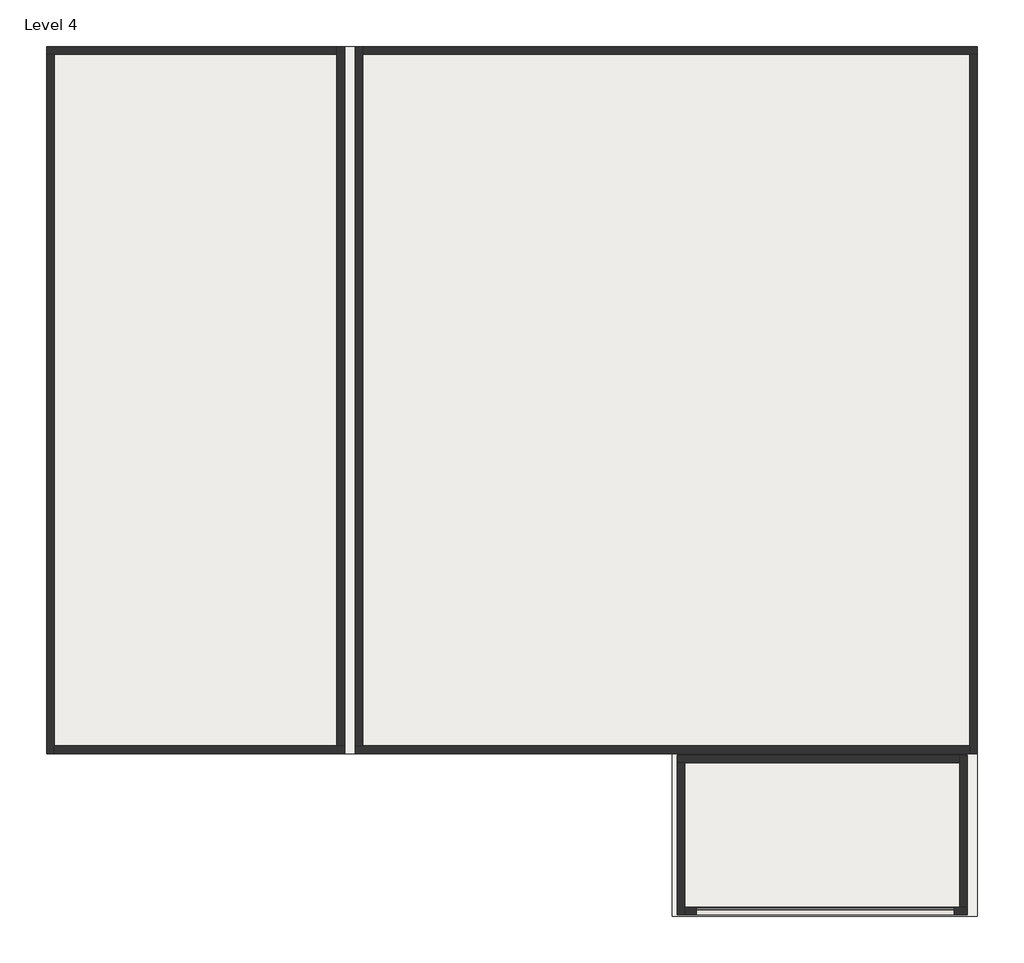
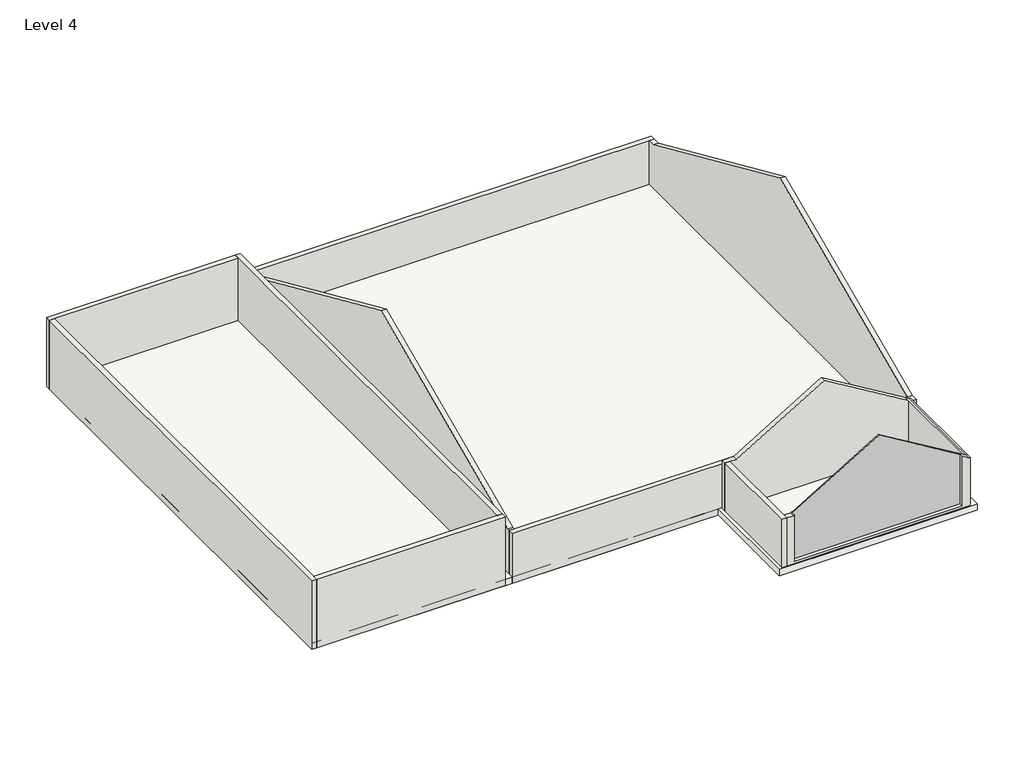
# One storey: 12 walls, 1 plate, 1 slab.
"""IFC4 building model written with IfcOpenShell, lengths in millimetres."""

from ifc_helpers import new_model, si_unit, frame, origin, place, context, project, spatial, polyline, outline, extrude, faceted_brep, transform, mapped, element, save
from components import system_panel_glazed_24e5f3e2

model = new_model("IFC4")

# Units and contexts
model_context = context("Model", 3, world=origin())
ifc_project = project(units=[si_unit("LENGTHUNIT", "METRE", prefix="MILLI")], contexts=[model_context])

# Site, building, storey
site = spatial("IfcSite", under=ifc_project)
building = spatial("IfcBuilding", under=site)
storey = spatial("IfcBuildingStorey", under=building, Name="Level 4", Elevation=6858.0)

# Plate
placement = place(None, origin())
system_panel_glazed_shape = system_panel_glazed_24e5f3e2(model_context)
element("IfcPlate", 1, ObjectType="System Panel : Glazed", at=placement, inside=storey, context=model_context, shape_type="MappedRepresentation", body=[
    mapped(system_panel_glazed_shape, transform((5277.9635732, -1650.5734736, 7068.8144542), x_axis=(1.0, 0.0, 0.0), y_axis=(0.0, 1.0, 0.0), z_axis=(0.0, 0.0, 1.0))),
])

# Slab
element("IfcSlab", 2, ObjectType="6\" GF", at=placement, inside=storey, context=model_context, shape_type="SweptSolid", body=[
    extrude(outline(polyline([(-6386.9864268, 11297.0765264), (7557.6135732, 11297.0765264), (7557.6135732, -1733.1234736), (2985.6135732, -1733.1234736), (2985.6135732, 705.2765264), (365.6851234, 705.2765264), (-6386.9864268, 705.2765264), (-6386.9864268, 11297.0765264)])), frame((0.0, 0.0, 6858.0), z_axis=(0.0, 0.0, 1.0), x_axis=(1.0, 0.0, 0.0)), (0.0, 0.0, 1.0), 152.4),
])

# Walls
element("IfcWall", 3, ObjectType="4.5\" wall", at=placement, inside=storey, context=model_context, shape_type="Brep", body=[
    faceted_brep([(7405.2135732, -1593.4234736, 6858.0), (7290.9135732, -1593.4234736, 6858.0), (3176.1135732, -1593.4234736, 6858.0), (3176.1135732, -1593.4234736, 8183.7639477), (3326.968548, -1593.4234736, 8183.7639477), (3347.5635732, -1593.4234736, 8196.1386873), (3347.5635732, -1593.4234736, 7068.8144542), (7208.3635732, -1593.4234736, 7068.8144542), (7208.3635732, -1593.4234736, 8280.0789158), (7290.9135732, -1593.4234736, 8230.4778717), (7368.6585985, -1593.4234736, 8183.7639477), (7405.2135732, -1593.4234736, 8183.7639477), (3176.1135732, -1707.7234736, 6858.0), (7405.2135732, -1707.7234736, 6858.0), (7405.2135732, -1707.7234736, 8183.7639477), (7368.6585985, -1707.7234736, 8183.7639477), (7208.3635732, -1707.7234736, 8280.0789158), (7208.3635732, -1707.7234736, 7068.8144542), (3347.5635732, -1707.7234736, 7068.8144542), (3347.5635732, -1707.7234736, 8196.1386873), (3326.968548, -1707.7234736, 8183.7639477), (3176.1135732, -1707.7234736, 8183.7639477)], [[[0, 1, 2, 3, 4, 5, 6, 7, 8, 9, 10, 11]], [[12, 13, 14, 15, 16, 17, 18, 19, 20, 21]], [[2, 1, 0, 13, 12]], [[0, 11, 14, 13]], [[3, 2, 12, 21]], [[14, 11, 10, 15]], [[15, 10, 9, 8, 16]], [[4, 20, 19, 5]], [[3, 21, 20, 4]], [[18, 6, 5, 19]], [[7, 17, 16, 8]], [[6, 18, 17, 7]]]),
])
element("IfcWall", 4, ObjectType="4.5\" wall", at=placement, inside=storey, context=model_context, shape_type="Brep", body=[
    faceted_brep([(7290.9135732, 679.8765264, 6858.0), (7290.9135732, 565.5765264, 6858.0), (7290.9135732, -1593.4234736, 6858.0), (7290.9135732, -1593.4234736, 8230.4778717), (7290.9135732, 565.5765264, 8230.4778717), (7290.9135732, 679.8765264, 8230.4778717), (7405.2135732, 679.8765264, 6858.0), (7405.2135732, 679.8765264, 8183.7639477), (7405.2135732, -1593.4234736, 8183.7639477), (7405.2135732, -1593.4234736, 6858.0), (7368.6585985, 679.8765264, 8183.7639477), (7368.6585985, -1593.4234736, 8183.7639477)], [[[0, 1, 2, 3, 4, 5]], [[6, 7, 8, 9]], [[2, 1, 0, 6, 9]], [[0, 5, 10, 7, 6]], [[3, 2, 9, 8, 11]], [[5, 4, 3, 11, 10]], [[11, 8, 7, 10]]]),
])
element("IfcWall", 5, ObjectType="4.5\" wall", at=placement, inside=storey, context=model_context, shape_type="Brep", body=[
    faceted_brep([(3061.8135732, 565.5765264, 6858.0), (3176.1135732, 565.5765264, 6858.0), (7290.9135732, 565.5765264, 6858.0), (7290.9135732, 565.5765264, 8230.4778717), (5347.8135732, 565.5765264, 9398.0101405), (3326.968548, 565.5765264, 8183.7639477), (3176.1135732, 565.5765264, 8183.7639477), (3061.8135732, 565.5765264, 8183.7639477), (3061.8135732, 679.8765264, 6858.0), (3061.8135732, 679.8765264, 8183.7639477), (3326.968548, 679.8765264, 8183.7639477), (5347.8135732, 679.8765264, 9398.0101405), (7290.9135732, 679.8765264, 8230.4778717), (7290.9135732, 679.8765264, 6858.0)], [[[0, 1, 2, 3, 4, 5, 6, 7]], [[8, 9, 10, 11, 12, 13]], [[2, 1, 0, 8, 13]], [[0, 7, 9, 8]], [[3, 2, 13, 12]], [[7, 6, 5, 10, 9]], [[5, 4, 11, 10]], [[4, 3, 12, 11]]]),
])
element("IfcWall", 6, ObjectType="4.5\" wall", at=placement, inside=storey, context=model_context, shape_type="Brep", body=[
    faceted_brep([(3176.1135732, -1707.7234736, 6858.0), (3176.1135732, -1593.4234736, 6858.0), (3176.1135732, 565.5765264, 6858.0), (3176.1135732, 565.5765264, 8183.7639477), (3176.1135732, -1593.4234736, 8183.7639477), (3176.1135732, -1707.7234736, 8183.7639477), (3061.8135732, -1707.7234736, 6858.0), (3061.8135732, -1707.7234736, 8183.7639477), (3061.8135732, 565.5765264, 8183.7639477), (3061.8135732, 565.5765264, 6858.0)], [[[0, 1, 2, 3, 4, 5]], [[6, 7, 8, 9]], [[2, 1, 0, 6, 9]], [[0, 5, 7, 6]], [[3, 2, 9, 8]], [[5, 4, 3, 8, 7]]]),
])
element("IfcWall", 7, ObjectType="4.5\" wall", at=placement, inside=storey, context=model_context, shape_type="Brep", body=[
    faceted_brep([(7557.6135732, 11297.0765264, 6858.0), (-1648.9651673, 11297.0765264, 6858.0), (-1648.9651673, 11297.0765264, 8077.2), (7557.6135732, 11297.0765264, 8077.2), (7557.6135732, 11182.7765264, 6858.0), (7557.6135732, 11182.7765264, 8077.2), (7443.3135732, 11182.7765264, 8077.2), (-1648.9651673, 11182.7765264, 8077.2), (-1648.9651673, 11182.7765264, 6858.0), (7443.3135732, 11182.7765264, 6858.0)], [[[0, 1, 2, 3]], [[4, 5, 6, 7, 8, 9]], [[1, 0, 4, 9, 8]], [[3, 2, 7, 6, 5]], [[0, 3, 5, 4]], [[2, 1, 8, 7]]]),
])
element("IfcWall", 8, ObjectType="4.5\" wall", at=placement, inside=storey, context=model_context, shape_type="Brep", body=[
    faceted_brep([(7557.6135732, 705.2765264, 6858.0), (7557.6135732, 11182.7765264, 6858.0), (7557.6135732, 11182.7765264, 8077.2), (7557.6135732, 11013.6793515, 8077.2), (7557.6135732, 5944.0265264, 10334.3548623), (7557.6135732, 874.3737012, 8077.2), (7557.6135732, 705.2765264, 8077.2), (7443.3135732, 705.2765264, 6858.0), (7443.3135732, 705.2765264, 8077.2), (7443.3135732, 819.5765264, 8077.2), (7443.3135732, 874.3737012, 8077.2), (7443.3135732, 5944.0265264, 10334.3548623), (7443.3135732, 11013.6793515, 8077.2), (7443.3135732, 11182.7765264, 8077.2), (7443.3135732, 11182.7765264, 6858.0), (7443.3135732, 819.5765264, 6858.0)], [[[0, 1, 2, 3, 4, 5, 6]], [[7, 8, 9, 10, 11, 12, 13, 14, 15]], [[1, 0, 7, 15, 14]], [[0, 6, 8, 7]], [[2, 1, 14, 13]], [[6, 5, 10, 9, 8]], [[5, 4, 11, 10]], [[4, 3, 12, 11]], [[3, 2, 13, 12]]]),
])
element("IfcWall", 9, ObjectType="4.5\" wall", at=placement, inside=storey, context=model_context, shape_type="Brep", body=[
    faceted_brep([(-1763.2651673, 705.2765264, 6858.0), (7443.3135732, 705.2765264, 6858.0), (7443.3135732, 705.2765264, 8077.2), (-1763.2651673, 705.2765264, 8077.2), (-1763.2651673, 819.5765264, 6858.0), (-1763.2651673, 819.5765264, 8077.2), (-1648.9651673, 819.5765264, 8077.2), (7443.3135732, 819.5765264, 8077.2), (7443.3135732, 819.5765264, 6858.0), (-1648.9651673, 819.5765264, 6858.0)], [[[0, 1, 2, 3]], [[4, 5, 6, 7, 8, 9]], [[1, 0, 4, 9, 8]], [[3, 2, 7, 6, 5]], [[0, 3, 5, 4]], [[2, 1, 8, 7]]]),
])
element("IfcWall", 10, ObjectType="4.5\" wall", at=placement, inside=storey, context=model_context, shape_type="Brep", body=[
    faceted_brep([(-1763.2651673, 11297.0765264, 6858.0), (-1763.2651673, 819.5765264, 6858.0), (-1763.2651673, 819.5765264, 8077.2), (-1763.2651673, 874.3737012, 8077.2), (-1763.2651673, 5944.0265264, 10334.3548623), (-1763.2651673, 11013.6793515, 8077.2), (-1763.2651673, 11297.0765264, 8077.2), (-1648.9651673, 11297.0765264, 6858.0), (-1648.9651673, 11297.0765264, 8077.2), (-1648.9651673, 11182.7765264, 8077.2), (-1648.9651673, 11013.6793515, 8077.2), (-1648.9651673, 5944.0265264, 10334.3548623), (-1648.9651673, 874.3737012, 8077.2), (-1648.9651673, 819.5765264, 8077.2), (-1648.9651673, 819.5765264, 6858.0), (-1648.9651673, 11182.7765264, 6858.0)], [[[0, 1, 2, 3, 4, 5, 6]], [[7, 8, 9, 10, 11, 12, 13, 14, 15]], [[1, 0, 7, 15, 14]], [[0, 6, 8, 7]], [[2, 1, 14, 13]], [[6, 5, 10, 9, 8]], [[5, 4, 11, 10]], [[4, 3, 12, 11]], [[3, 2, 13, 12]]]),
])
element("IfcWall", 11, ObjectType="4.5\" wall", at=placement, inside=storey, context=model_context, shape_type="Brep", body=[
    faceted_brep([(-6386.9864268, 11182.7765264, 6858.0), (-6272.6864268, 11182.7765264, 6858.0), (-2037.3924436, 11182.7765264, 6858.0), (-2037.3924436, 11182.7765264, 8533.9641574), (-6272.6864268, 11182.7765264, 8533.9641574), (-6386.9864268, 11182.7765264, 8533.9641574), (-6386.9864268, 11297.0765264, 6858.0), (-6386.9864268, 11297.0765264, 8533.9641574), (-2037.3924436, 11297.0765264, 8533.9641574), (-2037.3924436, 11297.0765264, 6858.0)], [[[0, 1, 2, 3, 4, 5]], [[6, 7, 8, 9]], [[2, 1, 0, 6, 9]], [[5, 4, 3, 8, 7]], [[0, 5, 7, 6]], [[3, 2, 9, 8]]]),
])
element("IfcWall", 12, ObjectType="4.5\" wall", at=placement, inside=storey, context=model_context, shape_type="Brep", body=[
    faceted_brep([(-6272.6864268, 705.2765264, 6858.0), (-6272.6864268, 819.5765264, 6858.0), (-6272.6864268, 11182.7765264, 6858.0), (-6272.6864268, 11182.7765264, 8533.9641574), (-6272.6864268, 819.5765264, 8533.9641574), (-6272.6864268, 705.2765264, 8533.9641574), (-6386.9864268, 705.2765264, 6858.0), (-6386.9864268, 705.2765264, 8533.9641574), (-6386.9864268, 11182.7765264, 8533.9641574), (-6386.9864268, 11182.7765264, 6858.0)], [[[0, 1, 2, 3, 4, 5]], [[6, 7, 8, 9]], [[2, 1, 0, 6, 9]], [[5, 4, 3, 8, 7]], [[0, 5, 7, 6]], [[3, 2, 9, 8]]]),
])
element("IfcWall", 13, ObjectType="4.5\" wall", at=placement, inside=storey, context=model_context, shape_type="Brep", body=[
    faceted_brep([(-1923.0924436, 819.5765264, 6858.0), (-2037.3924436, 819.5765264, 6858.0), (-6272.6864268, 819.5765264, 6858.0), (-6272.6864268, 819.5765264, 8533.9641574), (-2037.3924436, 819.5765264, 8533.9641574), (-1923.0924436, 819.5765264, 8533.9641574), (-1923.0924436, 705.2765264, 6858.0), (-1923.0924436, 705.2765264, 8533.9641574), (-6272.6864268, 705.2765264, 8533.9641574), (-6272.6864268, 705.2765264, 6858.0)], [[[0, 1, 2, 3, 4, 5]], [[6, 7, 8, 9]], [[2, 1, 0, 6, 9]], [[5, 4, 3, 8, 7]], [[0, 5, 7, 6]], [[3, 2, 9, 8]]]),
])
element("IfcWall", 14, ObjectType="4.5\" wall", at=placement, inside=storey, context=model_context, shape_type="Brep", body=[
    faceted_brep([(-2037.3924436, 11297.0765264, 6858.0), (-2037.3924436, 11182.7765264, 6858.0), (-2037.3924436, 819.5765264, 6858.0), (-2037.3924436, 819.5765264, 8533.9641574), (-2037.3924436, 11182.7765264, 8533.9641574), (-2037.3924436, 11297.0765264, 8533.9641574), (-1923.0924436, 11297.0765264, 6858.0), (-1923.0924436, 11297.0765264, 8533.9641574), (-1923.0924436, 819.5765264, 8533.9641574), (-1923.0924436, 819.5765264, 6858.0)], [[[0, 1, 2, 3, 4, 5]], [[6, 7, 8, 9]], [[2, 1, 0, 6, 9]], [[5, 4, 3, 8, 7]], [[0, 5, 7, 6]], [[3, 2, 9, 8]]]),
])

save(model, "model.ifc")

# Revit data of these elements
# Type "System Panel : Glazed"
#   Construction Type Id = "GSP4R"
#   Analytic Construction = "1/8 in Pilkington single glazing"
#   Visual Light Transmittance = 0.9
#   Solar Heat Gain Coefficient = 0.86
#   Heat Transfer Coefficient (U) = 1.18115 BTU/(h·ft²·°F)
#   Define Thermal Properties by = 1
# Type "6\" GF"
#   Assembly Code = "B1010"
#   Function = 0
#   Layers, outside or top first: 0' - 6" "wall" (function 1)
# Type "4.5\" wall"
#   Assembly Code = "B2010"
#   Layers, outside or top first: 0' - 4 1/2" "Gypsum Wall Board" (function 1)
# Element 1 (IfcPlate, "System Panel : Glazed")
#   Phase Created = New Construction
#   Materials on its faces: "Glass"
# Element 2 (IfcSlab, "6\" GF")
#   built-in parameter 1001955 = 3.14159 (stored number, unit not read)
#   Height Offset From Level = 0' - 6"
#   Phase Created = New Construction
#   Materials on its faces: "wall"
# Elements 3, 4, 5, 6 (IfcWall, "4.5\" wall")
#   Top Offset = 0' - 0"
#   Base Offset = 0' - 0"
#   wall height = 4' - 0"
#   Phase Created = New Construction
#   Base Constraint = Level 4
#   Top Constraint = Level 5
#   Materials on its faces: "Gypsum Wall Board"
# Elements 7, 8, 9, 10 (IfcWall, "4.5\" wall")
#   Top Offset = 0' - 0"
#   Base Offset = 0' - 0"
#   Unconnected Height = 4' - 0"
#   wall height = 4' - 0"
#   Phase Created = New Construction
#   Base Constraint = Level 4
#   Materials on its faces: "Gypsum Wall Board"
# Elements 11, 12, 13, 14 (IfcWall, "4.5\" wall")
#   Top Offset = 0' - 0"
#   Base Offset = 0' - 0"
#   Unconnected Height = 5' - 5.98284"
#   wall height = 5' - 5.98284"
#   Phase Created = New Construction
#   Base Constraint = Level 4
#   Materials on its faces: "Gypsum Wall Board"
# Materials
#   "wall": class "Generic", colour RGB 120 120 120, transparency 0, Cost = 0
#   "Gypsum Wall Board": class "Generic", colour RGB 127 127 127, transparency 0, Description = "Gypsum Wall Board", Cost = 0
#   "Glass": class "Glass", colour RGB 0 128 192, transparency 0.75, Description = "Soda Lime Glass", Cost = 0
